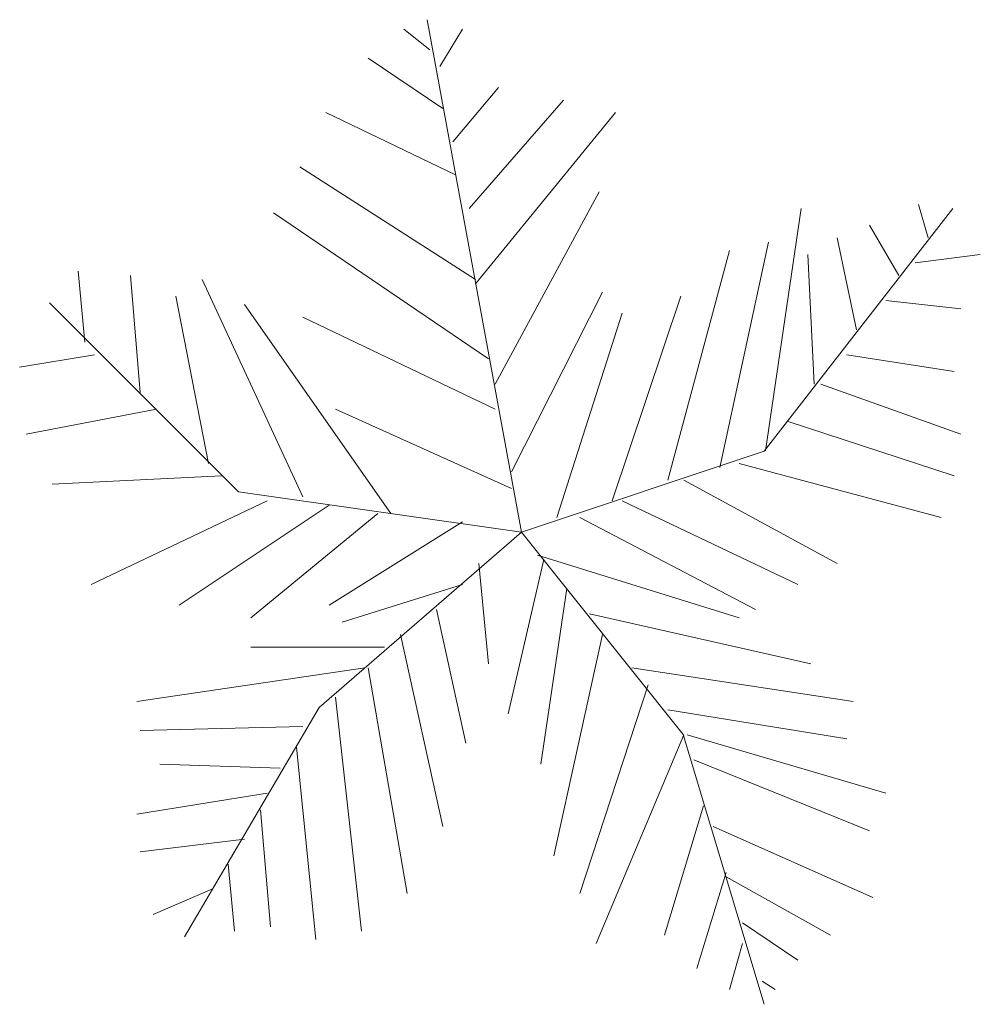
# Model space of a CAD drawing. Units: inches. Extents: x 177 to 1423, y 532 to 2503.
# Tile 5 of 5: x 1410.61 to 1422.55, y 2490.98 to 2503.21. Entities that reach past the tile are written whole.
import ezdxf

# ---------------------------------------------------------------- set-up
doc = ezdxf.new("R2010")
doc.units = ezdxf.units.IN
doc.layers.add('L-PLNT', color=94, linetype='Continuous', lineweight=13)

# ---------------------------------------------------------------- blocks, each defined once
blk = doc.blocks.new('*U11')
for p, q in [((0, 0), (-10.5, 57)), ((-10.186, 53.64), (-13.084, 55.962)), ((-9.099, 51.782), (-6.563, 55.962)), ((-8.737, 47.138), (-17.069, 52.711)), ((-7.65, 43.423), (-2.578, 49.46)), ((-5.839, 35.992), (4.667, 48.067)), ((-7.288, 39.707), (-21.778, 46.673)), ((-5.114, 27.632), (10.463, 46.673)), ((-5.114, 28.097), (-24.676, 40.636)), ((-2.941, 16.486), (8.652, 37.85)), ((44.153, 36.456), (45.239, 32.741)), ((-3.665, 19.273), (-27.574, 35.527)), ((27, 9), (48, 36)), ((27.127, 9.056), (31.112, 35.992)), ((38.719, 34.134), (41.979, 28.561)), ((22.055, 7.198), (27.489, 32.277)), ((35.096, 32.741), (37.27, 22.524)), ((16.259, 5.805), (23.142, 31.348)), ((31.836, 30.883), (32.561, 16.486)), ((43.791, 29.954), (51.036, 30.883)), ((-48.585, 21.131), (-49.309, 29.026)), ((-43.513, 28.561), (-42.427, 15.558)), ((-35.544, 28.097), (-24.314, 3.947)), ((-1.129, 6.734), (9.014, 26.704)), ((-31.5, 4.5), (-52.5, 25.5)), ((-38.442, 26.239), (-34.819, 7.663)), ((-14.533, 2.09), (-30.834, 25.31)), ((10.101, 3.483), (17.708, 26.239)), ((40.53, 25.775), (48.862, 24.846)), ((3.942, 1.625), (11.187, 24.381)), ((-24.314, 23.917), (-2.941, 13.7)), ((-47.498, 19.737), (-55.83, 18.344)), ((36.183, 19.737), (48.137, 17.88)), ((33.285, 16.486), (48.862, 10.913)), ((-40.615, 13.7), (-55.105, 10.913)), ((-20.691, 13.7), (-1.129, 4.876)), ((29.662, 12.307), (48.137, 6.269)), ((0, 0), (27, 9)), ((24.229, 7.663), (46.688, 1.625)), ((-33.37, 6.269), (-52.207, 5.34)), ((18.07, 5.805), (35.096, -3.483)), ((0, 0), (-31.5, 4.5)), ((-28.299, 3.483), (-47.86, -5.805)), ((11.187, 3.483), (30.749, -5.805)), ((-21.416, 3.018), (-38.079, -8.128)), ((-15.982, 2.09), (-30.11, -9.521)), ((-6.563, 1.161), (-21.416, -8.128)), ((6.478, 1.625), (26.04, -8.592)), ((0, 0), (-22.5, -19.5)), ((0, 0), (18, -22.5)), ((2.493, -3.019), (-1.491, -20.202)), ((1.769, -2.555), (24.229, -9.521)), ((-4.752, -3.483), (-3.665, -14.629)), ((-6.563, -5.805), (-19.967, -9.985)), ((5.029, -6.27), (2.131, -25.775)), ((-9.461, -8.592), (-6.201, -23.453)), ((7.565, -9.056), (32.198, -14.629)), ((-13.446, -11.378), (-8.737, -32.741)), ((9.014, -11.378), (3.58, -35.992)), ((-15.257, -12.772), (-30.11, -12.772)), ((-17.431, -15.094), (-42.789, -18.809)), ((-17.069, -15.094), (-12.721, -40.172)), ((12.274, -15.094), (36.907, -18.809)), ((14.085, -16.951), (6.478, -40.172)), ((-20.691, -18.345), (-17.793, -44.352)), ((-22.5, -19.5), (-37.5, -45)), ((16.259, -19.738), (36.183, -22.989)), ((-24.314, -21.596), (-42.427, -22.06)), ((18.07, -22.524), (8.289, -45.745)), ((18, -22.5), (27, -52.5)), ((18.433, -22.524), (40.53, -29.026)), ((-25.038, -23.918), (-22.865, -45.281)), ((-26.849, -26.24), (-40.253, -25.775)), ((19.157, -25.311), (38.719, -33.206)), ((-28.299, -29.026), (-42.789, -31.348)), ((20.244, -30.419), (15.897, -44.816)), ((-29.023, -30.884), (-27.936, -43.887)), ((21.331, -32.741), (39.081, -40.636)), ((-30.834, -34.135), (-42.427, -35.528)), ((-32.646, -36.921), (-31.921, -44.352)), ((22.78, -37.85), (19.519, -48.532)), ((22.78, -38.314), (34.372, -44.816)), ((-34.457, -39.708), (-40.978, -42.494)), ((24.591, -43.423), (30.749, -47.603)), ((24.591, -45.745), (23.142, -50.854)), ((26.764, -49.925), (28.213, -50.854))]:
    blk.add_line(p, q)

msp = doc.modelspace()

# ---------------------------------------------------------------- block references
at = {"layer": 'L-PLNT', "xscale": 0.1117025751797268, "yscale": 0.1117025751797268, "zscale": 0.1117025751797268}
msp.add_blockref('*U11', (1416.847, 2496.84), dxfattribs=at)

doc.saveas('drawing.dxf')
